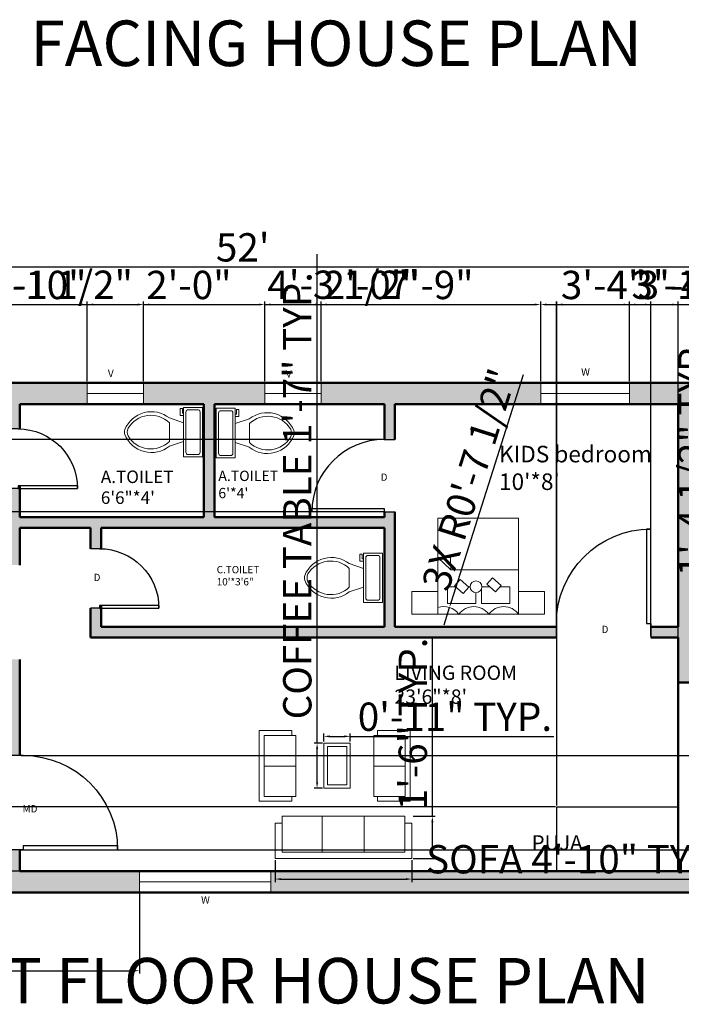
# Model space of a CAD drawing. Units: inches. Extents: x 2225 to 3094, y 1739 to 2599.
# Tile 3 of 5: x 2500 to 2780, y 2171 to 2588. Entities that reach past the tile are written whole.
import ezdxf

# ---------------------------------------------------------------- set-up
doc = ezdxf.new("R2010")
doc.units = ezdxf.units.IN
for name, color, linetype, lineweight in [('A-ANNO-DIMS', 2, 'Continuous', 18), ('A-ANNO-TEXT', 7, 'Continuous', 18), ('A-ANNO-TITL', 7, 'Continuous', 35), ('A-AREA-IDEN', 7, 'Continuous', 18), ('A-DOOR', 4, 'Continuous', 25), ('A-FLOR-CASE', 9, 'Continuous', 25), ('A-FLOR-FIXT', 9, 'Continuous', 18), ('A-FURN', 8, 'Continuous', 18), ('A-WALL-PATT', 160, 'Continuous', 13), ('WALL', 7, 'Continuous', 50), ('WINDOW', 130, 'Continuous', 18)]:
    doc.layers.add(name, color=color, linetype=linetype, lineweight=lineweight)
doc.styles.get("Standard").update_dxf_attribs({"font": 'arial.ttf'})
doc.dimstyles.new('ISO-25', dxfattribs={"dimtxt": 12, "dimasz": 2.5, "dimexe": 1.25, "dimexo": 0.625, "dimtad": 1, "dimdec": 0, "dimlunit": 4, "dimtxsty": 'Standard', "dimcen": 2.5, "dimadec": 0, "dimazin": 0, "dimtfac": 1, "dimtdec": 0, "dimtmove": 0, "dimatfit": 3, "dimfxl": 1, "dimarcsym": 0})

# ---------------------------------------------------------------- blocks, each defined once
blk = doc.blocks.new('*U2')
for p, q in [((9.5, -6), (9.5, -2)), ((-8, -8.5), (-8, -8)), ((-7, -8), (-7, -9.5)), ((-4, -8), (-6, -14)), ((4, -8), (6, -14)), ((-10, -8.5), (-8, -8.5)), ((-10, -9.5), (-10, -8.5)), ((-7, -9.5), (-10, -9.5)), ((4, -14), (-4, -14))]:
    blk.add_line(p, q)
blk.add_lwpolyline([(10.5, -8), (10.5, 0), (-10.5, 0), (-10.5, -8)], close=True)
for points in [[(-9.5, -2), (-9.5, -6)], [(8.5, -1), (-8.5, -1)], [(-8.5, -7), (8.5, -7)]]:
    blk.add_lwpolyline(points)
for centre, radius, start, end in [((-8.62, -1.88), 0.884, 81.8699, 188.1301), ((8.62, -1.88), 0.884, 351.8699, 98.1301), ((-8.62, -6.12), 0.884, 171.8699, 278.1301), ((8.62, -6.12), 0.884, 261.8699, 8.1301), ((3.52, -21.58), 12.17, 141.4691, 247.9714), ((4.2, -21.82), 11.33, 136.3677, 238.9468), ((-3.52, -21.58), 12.17, 292.0284, 38.5307), ((-4.2, -21.82), 11.33, 301.053, 43.6321), ((0, -27.88), 4, 245.7318, 294.2682), ((0, -29), 4, 254.8605, 285.1395)]:
    blk.add_arc(centre, radius, start, end)
blk = doc.blocks.new('*U4')
for p, q in [((0, 0), (0, -6)), ((40, 0), (40, -6))]:
    blk.add_line(p, q)
blk.add_lwpolyline([(0, 0), (0, 40), (1.75, 40), (1.75, 0)], close=True)
blk.add_arc((0, 0), 40, 0, 90)
blk = doc.blocks.new('*D5')
at = {"layer": 'A-ANNO-DIMS', "color": 0, "lineweight": -2, "transparency": 16777216}
for p, q in [((2282.56, 2434.95), (2282.56, 2484.67)), ((2285.06, 2483.42), (2904.06, 2483.42)), ((2906.56, 2434.95), (2906.56, 2484.67))]:
    blk.add_line(p, q, dxfattribs=at)
at = {"layer": 'A-ANNO-DIMS', "color": 0, "transparency": 16777216}
for points in [[(2285.06, 2483.83), (2285.06, 2483), (2282.56, 2483.42)], [(2904.06, 2483.83), (2904.06, 2483), (2906.56, 2483.42)]]:
    blk.add_solid(points, dxfattribs=at)
at = {"layer": 'Defpoints', "color": 0, "transparency": 16777216}
for p in [(2906.56, 2483.42), (2282.56, 2434.33), (2906.56, 2434.33)]:
    blk.add_point(p, dxfattribs=at)
at = {"layer": 'A-ANNO-DIMS', "color": 0, "transparency": 16777216, "insert": (2594.56, 2490.17), "char_height": 12, "attachment_point": 5}
blk.add_mtext("52'", dxfattribs=at)
blk = doc.blocks.new('BED-SINGLE')
for p, q in [((16.5, 18.81), (10.96, 24.02)), ((10.96, 24.02), (16.28, 24.02)), ((16.28, 24.02), (16.5, 18.81)), ((45.21, 18.81), (16.5, 18.81))]:
    blk.add_line(p, q)
for points in [[(45.21, 0), (45.21, 40.75), (10.96, 40.75), (10.96, 0)], [(21.65, 8.84), (18.05, 12.11), (20.5, 14.81), (24.1, 11.54)], [(35.37, 9.52), (31.76, 12.79), (34.21, 15.49), (37.82, 12.22)], [(10.96, 0), (10.96, 9.73), (0, 9.73), (0, 0)], [(56.18, 0), (56.18, 9.73), (45.21, 9.73), (45.21, 0)]]:
    blk.add_lwpolyline(points, close=True)
for points in [[(18.53, 11.67), (15.12, 11.67), (15.12, 4.64), (27.15, 4.64), (27.15, 9.17)], [(24.65, 11.67), (23.96, 11.67)], [(29.45, 10.68), (29.45, 4.64), (41.48, 4.64), (41.48, 11.67), (37.32, 11.67)], [(32.99, 11.67), (29.65, 11.67)]]:
    blk.add_lwpolyline(points)
blk.add_circle((27.15, 11.67), 2.5)
for centre, end in [((13.6, -4.42), 109.9878), ((26.25, -4.42), 145.0719), ((38.89, -4.42), 145.0719)]:
    blk.add_arc(centre, 7.71, 34.9281, end)
blk = doc.blocks.new('SOFA-THREE-SEAT')
for p, q in [((19.92, 17.92), (19.92, 2.75)), ((37.66, 17.92), (37.66, 2.75)), ((3.02, 14.97), (0, 14.97)), ((0, 14.97), (0, 0)), ((57.91, 14.97), (54.99, 14.97)), ((57.91, 0), (57.91, 14.97)), ((0, 0), (57.91, 0))]:
    blk.add_line(p, q)
blk.add_lwpolyline([(3.02, 2.75), (54.99, 2.75), (54.99, 17.92), (3.02, 17.92)], close=True)
blk = doc.blocks.new('SOFA-TWO-SEAT')
for p, q in [((1.66, 27.74), (1.66, 29.95)), ((1.66, 29.95), (15.43, 29.95)), ((15.43, 29.95), (15.43, 0)), ((0, 14.84), (13.39, 14.84)), ((1.66, 0), (1.66, 1.94)), ((15.43, 0), (1.66, 0))]:
    blk.add_line(p, q)
blk.add_lwpolyline([(13.39, 1.94), (0, 1.94), (0, 27.74), (13.39, 27.74)], close=True)
blk = doc.blocks.new('TABLE-COFFEE')
for points in [[(0, 0), (11.17, 0), (11.17, 19.11), (0, 19.11)], [(1.5, 1.5), (9.67, 1.5), (9.67, 17.61), (1.5, 17.61)]]:
    blk.add_lwpolyline(points, close=True)
blk = doc.blocks.new('WIN-55P7IN')
blk.add_line((0, 4.5), (55.68, 4.5))
blk.add_lwpolyline([(0, 0), (55.68, 0), (55.68, 9), (0, 9)], close=True)
blk = doc.blocks.new('*D32')
at = {"layer": 'A-ANNO-DIMS', "color": 0, "lineweight": -2, "transparency": 16777216}
for p, q in [((2608.3, 2232.07), (2608.3, 2222.75)), ((2666.2, 2232.07), (2666.2, 2222.75)), ((2610.8, 2224), (2663.7, 2224)), ((2666.2, 2224), (2802.66, 2224))]:
    blk.add_line(p, q, dxfattribs=at)
at = {"layer": 'A-ANNO-DIMS', "color": 0, "transparency": 16777216}
for points in [[(2610.8, 2224.42), (2610.8, 2223.59), (2608.3, 2224)], [(2663.7, 2224.42), (2663.7, 2223.59), (2666.2, 2224)]]:
    blk.add_solid(points, dxfattribs=at)
at = {"layer": 'Defpoints', "color": 0, "transparency": 16777216}
for p in [(2608.3, 2232.69), (2666.2, 2232.69), (2666.2, 2224)]:
    blk.add_point(p, dxfattribs=at)
at = {"layer": 'A-ANNO-DIMS', "color": 0, "transparency": 16777216, "insert": (2735.68, 2230.84), "char_height": 12, "attachment_point": 5}
blk.add_mtext('SOFA 4\'-10" TYP.', dxfattribs=at)
blk = doc.blocks.new('*D33')
at = {"layer": 'A-ANNO-DIMS', "color": 0, "lineweight": -2, "transparency": 16777216}
for p, q in [((2674.89, 2250.61), (2674.89, 2326.38)), ((2666.83, 2250.61), (2676.14, 2250.61)), ((2674.89, 2235.19), (2674.89, 2248.11)), ((2666.83, 2232.69), (2676.14, 2232.69))]:
    blk.add_line(p, q, dxfattribs=at)
at = {"layer": 'A-ANNO-DIMS', "color": 0, "transparency": 16777216}
for points in [[(2674.47, 2248.11), (2675.31, 2248.11), (2674.89, 2250.61)], [(2674.47, 2235.19), (2675.31, 2235.19), (2674.89, 2232.69)]]:
    blk.add_solid(points, dxfattribs=at)
at = {"layer": 'Defpoints', "color": 0, "transparency": 16777216}
for p in [(2666.2, 2250.61), (2674.89, 2250.61), (2666.2, 2232.69)]:
    blk.add_point(p, dxfattribs=at)
at = {"layer": 'A-ANNO-DIMS', "color": 0, "transparency": 16777216, "insert": (2668.14, 2289.74), "char_height": 12, "attachment_point": 5, "rotation": 90}
blk.add_mtext('1\'-6" TYP.', dxfattribs=at)
blk = doc.blocks.new('*D36')
at = {"layer": 'A-ANNO-DIMS', "color": 0, "lineweight": -2, "transparency": 16777216}
for p, q in [((2626.06, 2281.62), (2626.06, 2488.79)), ((2628.3, 2281.62), (2624.81, 2281.62)), ((2626.06, 2265.01), (2626.06, 2279.12)), ((2628.3, 2262.51), (2624.81, 2262.51))]:
    blk.add_line(p, q, dxfattribs=at)
at = {"layer": 'A-ANNO-DIMS', "color": 0, "transparency": 16777216}
for points in [[(2625.65, 2279.12), (2626.48, 2279.12), (2626.06, 2281.62)], [(2625.65, 2265.01), (2626.48, 2265.01), (2626.06, 2262.51)]]:
    blk.add_solid(points, dxfattribs=at)
at = {"layer": 'Defpoints', "color": 0, "transparency": 16777216}
for p in [(2626.06, 2281.62), (2628.93, 2281.62), (2628.93, 2262.51)]:
    blk.add_point(p, dxfattribs=at)
at = {"layer": 'A-ANNO-DIMS', "color": 0, "transparency": 16777216, "insert": (2619.23, 2386.46), "char_height": 12, "attachment_point": 5, "rotation": 90}
blk.add_mtext('COFFEE TABLE 1\'-7" TYP.', dxfattribs=at)
blk = doc.blocks.new('*D37')
at = {"layer": 'A-ANNO-DIMS', "color": 0, "lineweight": -2, "transparency": 16777216}
for p, q in [((2628.93, 2282.25), (2628.93, 2285.74)), ((2631.43, 2284.49), (2637.6, 2284.49)), ((2640.1, 2282.25), (2640.1, 2285.74)), ((2640.1, 2284.49), (2726.32, 2284.49))]:
    blk.add_line(p, q, dxfattribs=at)
at = {"layer": 'A-ANNO-DIMS', "color": 0, "transparency": 16777216}
for points in [[(2631.43, 2284.9), (2631.43, 2284.07), (2628.93, 2284.49)], [(2637.6, 2284.9), (2637.6, 2284.07), (2640.1, 2284.49)]]:
    blk.add_solid(points, dxfattribs=at)
at = {"layer": 'Defpoints', "color": 0, "transparency": 16777216}
for p in [(2640.1, 2284.49), (2628.93, 2281.62), (2640.1, 2281.62)]:
    blk.add_point(p, dxfattribs=at)
at = {"layer": 'A-ANNO-DIMS', "color": 0, "transparency": 16777216, "insert": (2684.46, 2291.24), "char_height": 12, "attachment_point": 5}
blk.add_mtext('0\'-11" TYP.', dxfattribs=at)
blk = doc.blocks.new('*D39')
at = {"layer": 'A-ANNO-DIMS', "color": 0, "lineweight": -2, "transparency": 16777216}
for p, q in [((2793.48, 2349.95), (2793.48, 2453.67)), ((2796.79, 2349.95), (2792.23, 2349.95)), ((2793.48, 2335.78), (2793.48, 2347.45)), ((2796.79, 2333.28), (2792.23, 2333.28))]:
    blk.add_line(p, q, dxfattribs=at)
at = {"layer": 'A-ANNO-DIMS', "color": 0, "transparency": 16777216}
for points in [[(2793.06, 2347.45), (2793.89, 2347.45), (2793.48, 2349.95)], [(2793.06, 2335.78), (2793.89, 2335.78), (2793.48, 2333.28)]]:
    blk.add_solid(points, dxfattribs=at)
at = {"layer": 'Defpoints', "color": 0, "transparency": 16777216}
for p in [(2793.48, 2349.95), (2797.42, 2349.95), (2797.42, 2333.28)]:
    blk.add_point(p, dxfattribs=at)
at = {"layer": 'A-ANNO-DIMS', "color": 0, "transparency": 16777216, "insert": (2786.65, 2403.06), "char_height": 12, "attachment_point": 5, "rotation": 90}
blk.add_mtext('1\'-4 1/2" TYP.', dxfattribs=at)
blk = doc.blocks.new('*D55')
at = {"layer": 'A-ANNO-DIMS', "color": 0, "lineweight": -2, "transparency": 16777216}
for p, q in [((2445.16, 2434.95), (2445.16, 2468.73)), ((2447.66, 2467.48), (2480.26, 2467.48)), ((2482.76, 2434.95), (2482.76, 2468.73)), ((2482.76, 2467.48), (2546.36, 2467.48))]:
    blk.add_line(p, q, dxfattribs=at)
at = {"layer": 'A-ANNO-DIMS', "color": 0, "transparency": 16777216}
for points in [[(2447.66, 2467.89), (2447.66, 2467.06), (2445.16, 2467.48)], [(2480.26, 2467.89), (2480.26, 2467.06), (2482.76, 2467.48)]]:
    blk.add_solid(points, dxfattribs=at)
at = {"layer": 'Defpoints', "color": 0, "transparency": 16777216}
for p in [(2482.76, 2467.48), (2445.16, 2434.33), (2482.76, 2434.33)]:
    blk.add_point(p, dxfattribs=at)
at = {"layer": 'A-ANNO-DIMS', "color": 0, "transparency": 16777216, "insert": (2515.81, 2474.31), "char_height": 12, "attachment_point": 5}
blk.add_mtext('3\'-1 1/2"', dxfattribs=at)
blk = doc.blocks.new('*D56')
at = {"layer": 'A-ANNO-DIMS', "color": 0, "lineweight": -2, "transparency": 16777216}
for p, q in [((2482.76, 2434.95), (2482.76, 2468.73)), ((2485.26, 2467.48), (2526.19, 2467.48)), ((2528.69, 2434.95), (2528.69, 2468.73))]:
    blk.add_line(p, q, dxfattribs=at)
at = {"layer": 'A-ANNO-DIMS', "color": 0, "transparency": 16777216}
for points in [[(2485.26, 2467.89), (2485.26, 2467.06), (2482.76, 2467.48)], [(2526.19, 2467.89), (2526.19, 2467.06), (2528.69, 2467.48)]]:
    blk.add_solid(points, dxfattribs=at)
at = {"layer": 'Defpoints', "color": 0, "transparency": 16777216}
for p in [(2528.69, 2467.48), (2482.76, 2434.33), (2528.69, 2434.33)]:
    blk.add_point(p, dxfattribs=at)
at = {"layer": 'A-ANNO-DIMS', "color": 0, "transparency": 16777216, "insert": (2505.72, 2474.23), "char_height": 12, "attachment_point": 5}
blk.add_mtext('3\'-10"', dxfattribs=at)
blk = doc.blocks.new('*D57')
at = {"layer": 'A-ANNO-DIMS', "color": 0, "lineweight": -2, "transparency": 16777216}
for p, q in [((2528.69, 2434.95), (2528.69, 2468.73)), ((2531.19, 2467.48), (2550.05, 2467.48)), ((2552.55, 2434.95), (2552.55, 2468.73)), ((2552.55, 2467.48), (2588.4, 2467.48))]:
    blk.add_line(p, q, dxfattribs=at)
at = {"layer": 'A-ANNO-DIMS', "color": 0, "transparency": 16777216}
for points in [[(2531.19, 2467.89), (2531.19, 2467.06), (2528.69, 2467.48)], [(2550.05, 2467.89), (2550.05, 2467.06), (2552.55, 2467.48)]]:
    blk.add_solid(points, dxfattribs=at)
at = {"layer": 'Defpoints', "color": 0, "transparency": 16777216}
for p in [(2552.55, 2467.48), (2528.69, 2434.33), (2552.55, 2434.33)]:
    blk.add_point(p, dxfattribs=at)
at = {"layer": 'A-ANNO-DIMS', "color": 0, "transparency": 16777216, "insert": (2571.73, 2474.23), "char_height": 12, "attachment_point": 5}
blk.add_mtext('2\'-0"', dxfattribs=at)
blk = doc.blocks.new('*D58')
at = {"layer": 'A-ANNO-DIMS', "color": 0, "lineweight": -2, "transparency": 16777216}
for p, q in [((2552.55, 2434.95), (2552.55, 2468.73)), ((2555.05, 2467.48), (2601.38, 2467.48)), ((2603.88, 2434.95), (2603.88, 2468.73)), ((2603.88, 2467.48), (2667.97, 2467.48))]:
    blk.add_line(p, q, dxfattribs=at)
at = {"layer": 'A-ANNO-DIMS', "color": 0, "transparency": 16777216}
for points in [[(2555.05, 2467.89), (2555.05, 2467.06), (2552.55, 2467.48)], [(2601.38, 2467.89), (2601.38, 2467.06), (2603.88, 2467.48)]]:
    blk.add_solid(points, dxfattribs=at)
at = {"layer": 'Defpoints', "color": 0, "transparency": 16777216}
for p in [(2603.88, 2467.48), (2552.55, 2434.33), (2603.88, 2434.33)]:
    blk.add_point(p, dxfattribs=at)
at = {"layer": 'A-ANNO-DIMS', "color": 0, "transparency": 16777216, "insert": (2637.18, 2474.31), "char_height": 12, "attachment_point": 5}
blk.add_mtext('4\'-3 1/2"', dxfattribs=at)
blk = doc.blocks.new('*D59')
at = {"layer": 'A-ANNO-DIMS', "color": 0, "lineweight": -2, "transparency": 16777216}
for p, q in [((2603.88, 2434.95), (2603.88, 2468.73)), ((2606.38, 2467.48), (2625.24, 2467.48)), ((2627.74, 2434.95), (2627.74, 2468.73)), ((2627.74, 2467.48), (2663.6, 2467.48))]:
    blk.add_line(p, q, dxfattribs=at)
at = {"layer": 'A-ANNO-DIMS', "color": 0, "transparency": 16777216}
for points in [[(2606.38, 2467.89), (2606.38, 2467.06), (2603.88, 2467.48)], [(2625.24, 2467.89), (2625.24, 2467.06), (2627.74, 2467.48)]]:
    blk.add_solid(points, dxfattribs=at)
at = {"layer": 'Defpoints', "color": 0, "transparency": 16777216}
for p in [(2627.74, 2467.48), (2603.88, 2434.33), (2627.74, 2434.33)]:
    blk.add_point(p, dxfattribs=at)
at = {"layer": 'A-ANNO-DIMS', "color": 0, "transparency": 16777216, "insert": (2646.92, 2474.23), "char_height": 12, "attachment_point": 5}
blk.add_mtext('2\'-0"', dxfattribs=at)
blk = doc.blocks.new('*D60')
at = {"layer": 'A-ANNO-DIMS', "color": 0, "lineweight": -2, "transparency": 16777216}
for p, q in [((2627.74, 2434.95), (2627.74, 2468.73)), ((2630.24, 2467.48), (2718.29, 2467.48)), ((2720.79, 2434.95), (2720.79, 2468.73))]:
    blk.add_line(p, q, dxfattribs=at)
at = {"layer": 'A-ANNO-DIMS', "color": 0, "transparency": 16777216}
for points in [[(2630.24, 2467.89), (2630.24, 2467.06), (2627.74, 2467.48)], [(2718.29, 2467.89), (2718.29, 2467.06), (2720.79, 2467.48)]]:
    blk.add_solid(points, dxfattribs=at)
at = {"layer": 'Defpoints', "color": 0, "transparency": 16777216}
for p in [(2720.79, 2467.48), (2627.74, 2434.33), (2720.79, 2434.33)]:
    blk.add_point(p, dxfattribs=at)
at = {"layer": 'A-ANNO-DIMS', "color": 0, "transparency": 16777216, "insert": (2674.27, 2474.23), "char_height": 12, "attachment_point": 5}
blk.add_mtext('7\'-9"', dxfattribs=at)
blk = doc.blocks.new('*D61')
at = {"layer": 'A-ANNO-DIMS', "color": 0, "lineweight": -2, "transparency": 16777216}
for p, q in [((2720.79, 2434.95), (2720.79, 2468.73)), ((2723.29, 2467.48), (2755.89, 2467.48)), ((2758.39, 2434.95), (2758.39, 2468.73)), ((2758.39, 2467.48), (2821.99, 2467.48))]:
    blk.add_line(p, q, dxfattribs=at)
at = {"layer": 'A-ANNO-DIMS', "color": 0, "transparency": 16777216}
for points in [[(2723.29, 2467.89), (2723.29, 2467.06), (2720.79, 2467.48)], [(2755.89, 2467.89), (2755.89, 2467.06), (2758.39, 2467.48)]]:
    blk.add_solid(points, dxfattribs=at)
at = {"layer": 'Defpoints', "color": 0, "transparency": 16777216}
for p in [(2758.39, 2467.48), (2720.79, 2434.33), (2758.39, 2434.33)]:
    blk.add_point(p, dxfattribs=at)
at = {"layer": 'A-ANNO-DIMS', "color": 0, "transparency": 16777216, "insert": (2791.44, 2474.31), "char_height": 12, "attachment_point": 5}
blk.add_mtext('3\'-1 1/2"', dxfattribs=at)
blk = doc.blocks.new('*D62')
at = {"layer": 'A-ANNO-DIMS', "color": 0, "lineweight": -2, "transparency": 16777216}
for p, q in [((2758.39, 2434.95), (2758.39, 2468.73)), ((2760.89, 2467.48), (2799.04, 2467.48)), ((2801.54, 2434.95), (2801.54, 2468.73))]:
    blk.add_line(p, q, dxfattribs=at)
at = {"layer": 'A-ANNO-DIMS', "color": 0, "transparency": 16777216}
for points in [[(2760.89, 2467.89), (2760.89, 2467.06), (2758.39, 2467.48)], [(2799.04, 2467.89), (2799.04, 2467.06), (2801.54, 2467.48)]]:
    blk.add_solid(points, dxfattribs=at)
at = {"layer": 'Defpoints', "color": 0, "transparency": 16777216}
for p in [(2801.54, 2467.48), (2758.39, 2434.33), (2801.54, 2434.33)]:
    blk.add_point(p, dxfattribs=at)
at = {"layer": 'A-ANNO-DIMS', "color": 0, "transparency": 16777216, "insert": (2779.97, 2474.23), "char_height": 12, "attachment_point": 5}
blk.add_mtext('3\'-7"', dxfattribs=at)
blk = doc.blocks.new('*D66')
at = {"layer": 'A-ANNO-DIMS', "color": 0, "lineweight": -2, "transparency": 16777216}
for p, q in [((2282.56, 2217.7), (2282.56, 2183.93)), ((2550.8, 2217.7), (2550.8, 2183.93)), ((2285.06, 2185.18), (2548.3, 2185.18))]:
    blk.add_line(p, q, dxfattribs=at)
at = {"layer": 'A-ANNO-DIMS', "color": 0, "transparency": 16777216}
for points in [[(2285.06, 2185.59), (2285.06, 2184.76), (2282.56, 2185.18)], [(2548.3, 2185.59), (2548.3, 2184.76), (2550.8, 2185.18)]]:
    blk.add_solid(points, dxfattribs=at)
at = {"layer": 'Defpoints', "color": 0, "transparency": 16777216}
for p in [(2282.56, 2218.33), (2550.8, 2218.33), (2550.8, 2185.18)]:
    blk.add_point(p, dxfattribs=at)
at = {"layer": 'A-ANNO-DIMS', "color": 0, "transparency": 16777216, "insert": (2416.68, 2191.83), "char_height": 12, "attachment_point": 5}
blk.add_mtext('22\'-4"', dxfattribs=at)
blk = doc.blocks.new('*D68')
at = {"layer": 'A-ANNO-DIMS', "color": 0, "lineweight": -2, "transparency": 16777216}
for p, q in [((2500.68, 2276.4), (2940.96, 2276.4)), ((2939.71, 2273.9), (2939.71, 2238.9)), ((2500.68, 2236.4), (2940.96, 2236.4))]:
    blk.add_line(p, q, dxfattribs=at)
at = {"layer": 'A-ANNO-DIMS', "color": 0, "transparency": 16777216}
for points in [[(2939.29, 2273.9), (2940.12, 2273.9), (2939.71, 2276.4)], [(2939.29, 2238.9), (2940.12, 2238.9), (2939.71, 2236.4)]]:
    blk.add_solid(points, dxfattribs=at)
at = {"layer": 'Defpoints', "color": 0, "transparency": 16777216}
for p in [(2500.06, 2276.4), (2500.06, 2236.4), (2939.71, 2236.4)]:
    blk.add_point(p, dxfattribs=at)
at = {"layer": 'A-ANNO-DIMS', "color": 0, "transparency": 16777216, "insert": (2932.95, 2256.4), "char_height": 12, "attachment_point": 5, "rotation": 90}
blk.add_mtext('3\'-4"', dxfattribs=at)
blk = doc.blocks.new('*D70')
at = {"layer": 'A-ANNO-DIMS', "color": 0, "lineweight": -2, "transparency": 16777216}
for p, q in [((2727.43, 2326.95), (2727.43, 2468.73)), ((2729.93, 2467.48), (2764.93, 2467.48)), ((2767.43, 2326.95), (2767.43, 2468.73))]:
    blk.add_line(p, q, dxfattribs=at)
at = {"layer": 'A-ANNO-DIMS', "color": 0, "transparency": 16777216}
for points in [[(2729.93, 2467.89), (2729.93, 2467.06), (2727.43, 2467.48)], [(2764.93, 2467.89), (2764.93, 2467.06), (2767.43, 2467.48)]]:
    blk.add_solid(points, dxfattribs=at)
at = {"layer": 'Defpoints', "color": 0, "transparency": 16777216}
for p in [(2767.43, 2467.48), (2727.43, 2326.33), (2767.43, 2326.33)]:
    blk.add_point(p, dxfattribs=at)
at = {"layer": 'A-ANNO-DIMS', "color": 0, "transparency": 16777216, "insert": (2747.43, 2474.23), "char_height": 12, "attachment_point": 5}
blk.add_mtext('3\'-4"', dxfattribs=at)
blk = doc.blocks.new('*D72')
at = {"layer": 'A-ANNO-DIMS', "color": 0, "lineweight": -2, "transparency": 16777216}
for p, q in [((2249.41, 2410.28), (2249.41, 2474.1)), ((2653.84, 2410.28), (2248.16, 2410.28)), ((2249.41, 2382.17), (2249.41, 2407.78)), ((2653.84, 2379.67), (2248.16, 2379.67))]:
    blk.add_line(p, q, dxfattribs=at)
at = {"layer": 'A-ANNO-DIMS', "color": 0, "transparency": 16777216}
for points in [[(2248.99, 2407.78), (2249.82, 2407.78), (2249.41, 2410.28)], [(2248.99, 2382.17), (2249.82, 2382.17), (2249.41, 2379.67)]]:
    blk.add_solid(points, dxfattribs=at)
at = {"layer": 'Defpoints', "color": 0, "transparency": 16777216}
for p in [(2249.41, 2410.28), (2654.47, 2410.28), (2654.47, 2379.67)]:
    blk.add_point(p, dxfattribs=at)
at = {"layer": 'A-ANNO-DIMS', "color": 0, "transparency": 16777216, "insert": (2242.58, 2443.44), "char_height": 12, "attachment_point": 5, "rotation": 90}
blk.add_mtext('2\'-6 1/2"', dxfattribs=at)
blk = doc.blocks.new('*D74')
at = {"layer": 'A-ANNO-DIMS', "color": 0, "lineweight": -2, "transparency": 16777216}
for p, q in [((2727.64, 2255.24), (2727.64, 2468.73)), ((2730.14, 2467.48), (2776.56, 2467.48)), ((2779.06, 2255.24), (2779.06, 2468.73)), ((2779.06, 2467.48), (2843.15, 2467.48))]:
    blk.add_line(p, q, dxfattribs=at)
at = {"layer": 'A-ANNO-DIMS', "color": 0, "transparency": 16777216}
for points in [[(2730.14, 2467.89), (2730.14, 2467.06), (2727.64, 2467.48)], [(2776.56, 2467.89), (2776.56, 2467.06), (2779.06, 2467.48)]]:
    blk.add_solid(points, dxfattribs=at)
at = {"layer": 'Defpoints', "color": 0, "transparency": 16777216}
for p in [(2779.06, 2467.48), (2727.64, 2254.61), (2779.06, 2254.61)]:
    blk.add_point(p, dxfattribs=at)
at = {"layer": 'A-ANNO-DIMS', "color": 0, "transparency": 16777216, "insert": (2812.35, 2474.31), "char_height": 12, "attachment_point": 5}
blk.add_mtext('4\'-3 1/2"', dxfattribs=at)
blk = doc.blocks.new('*D75')
at = {"layer": 'A-ANNO-DIMS', "color": 0, "lineweight": -2, "transparency": 16777216}
for p, q in [((2249.41, 2254.61), (2249.41, 2318.43)), ((2727.01, 2254.61), (2248.16, 2254.61)), ((2249.41, 2229.83), (2249.41, 2252.11)), ((2727.01, 2227.33), (2248.16, 2227.33))]:
    blk.add_line(p, q, dxfattribs=at)
at = {"layer": 'A-ANNO-DIMS', "color": 0, "transparency": 16777216}
for points in [[(2248.99, 2252.11), (2249.82, 2252.11), (2249.41, 2254.61)], [(2248.99, 2229.83), (2249.82, 2229.83), (2249.41, 2227.33)]]:
    blk.add_solid(points, dxfattribs=at)
at = {"layer": 'Defpoints', "color": 0, "transparency": 16777216}
for p in [(2249.41, 2254.61), (2727.64, 2254.61), (2727.64, 2227.33)]:
    blk.add_point(p, dxfattribs=at)
at = {"layer": 'A-ANNO-DIMS', "color": 0, "transparency": 16777216, "insert": (2242.57, 2287.77), "char_height": 12, "attachment_point": 5, "rotation": 90}
blk.add_mtext('2\'-3 1/2"', dxfattribs=at)
blk = doc.blocks.new('*D81')
at = {"layer": 'A-ANNO-DIMS', "color": 0, "lineweight": -2, "transparency": 16777216}
for p, q in [((2713.3, 2437.7), (2682.91, 2341.52)), ((2679.83, 2331.78), (2682.15, 2339.14))]:
    blk.add_line(p, q, dxfattribs=at)
at = {"layer": 'A-ANNO-DIMS', "color": 0, "transparency": 16777216}
blk.add_solid([(2682.51, 2341.65), (2683.3, 2341.39), (2682.15, 2339.14)], dxfattribs=at)
at = {"layer": 'Defpoints', "color": 0, "transparency": 16777216}
for p in [(2682.15, 2339.14), (2679.83, 2331.78)]:
    blk.add_point(p, dxfattribs=at)
at = {"layer": 'A-ANNO-DIMS', "color": 0, "transparency": 16777216, "insert": (2691.97, 2392.86), "char_height": 12, "attachment_point": 5, "rotation": 72.4604}
blk.add_mtext('3X R0\'-7 1/2"', dxfattribs=at)

msp = doc.modelspace()

# ---------------------------------------------------------------- hatches: boundary and pattern name
at = {"layer": 'A-WALL-PATT'}
h = msp.add_hatch(color=256, dxfattribs=at)
h.dxf.hatch_style = 1
h.paths.add_polyline_path([(2445.16, 2434.33), (2282.56, 2434.33), (2282.56, 2366.97), (2291.56, 2366.97), (2291.56, 2425.33), (2445.16, 2425.33)], flags=17)
h.paths.add_polyline_path([(2528.69, 2434.33), (2482.76, 2434.33), (2482.76, 2425.33), (2495.56, 2425.33), (2495.56, 2414.78), (2499.34, 2414.78, -0.007163), (2500.06, 2414.76), (2500.06, 2425.33), (2528.69, 2425.33)], flags=17)
h.paths.add_polyline_path([(2867.81, 2330.83), (2783.56, 2330.83), (2783.56, 2354.83), (2783.56, 2425.33), (2801.54, 2425.33), (2801.54, 2434.33), (2758.39, 2434.33), (2758.39, 2425.33), (2779.06, 2425.33), (2779.06, 2330.83), (2767.43, 2330.83), (2767.43, 2326.33), (2779.06, 2326.33), (2779.06, 2307.37), (2783.56, 2307.37), (2783.56, 2326.33), (2867.81, 2326.33)])
h.paths.add_polyline_path([(2906.56, 2434.33), (2839.14, 2434.33), (2839.14, 2425.33), (2897.56, 2425.33), (2897.56, 2330.83), (2897.56, 2326.33), (2897.56, 2264.13), (2906.56, 2264.13)])
h.paths.add_polyline_path([(2906.56, 2236.32), (2897.56, 2236.32), (2897.56, 2227.33), (2860.08, 2227.33), (2860.08, 2218.33), (2906.56, 2218.33)])
h.paths.add_polyline_path([(2815.14, 2227.33), (2783.56, 2227.33), (2779.06, 2227.33), (2727.64, 2227.33), (2606.48, 2227.33), (2606.48, 2218.33), (2815.14, 2218.33)])
h.paths.add_polyline_path([(2780.45, 2273.09), (2785.35, 2273.09), (2785.35, 2279.46), (2780.45, 2279.46)], flags=9)
h.paths.add_polyline_path([(2500.16, 2250.57), (2508.42, 2250.57), (2508.42, 2256.93), (2500.16, 2256.93)], flags=25)
h.paths.add_polyline_path([(2745.49, 2326.59), (2750.15, 2326.59), (2750.15, 2332.96), (2745.49, 2332.96)], flags=9)
h.paths.add_polyline_path([(2651.86, 2391.09), (2656.53, 2391.09), (2656.53, 2397.46), (2651.86, 2397.46)], flags=9)
h.paths.add_polyline_path([(2493.47, 2330.16), (2498.13, 2330.16), (2498.13, 2336.53), (2493.47, 2336.53)], flags=25)
h.paths.add_polyline_path([(2530.27, 2348.62), (2534.93, 2348.62), (2534.93, 2354.99), (2530.27, 2354.99)], flags=25)
h.paths.add_polyline_path([(2432.89, 2282.56), (2450.26, 2282.56), (2450.26, 2294.09), (2432.89, 2294.09)], flags=25)
h.paths.add_polyline_path([(2735.79, 2240.68), (2748.37, 2240.68), (2748.37, 2247.05), (2735.79, 2247.05)], flags=9)
h.paths.add_polyline_path([(2717.02, 2288.94), (2747.35, 2288.94), (2747.35, 2300.47), (2717.02, 2300.47)], flags=9)
h.paths.add_polyline_path([(2839.5, 2270.61), (2856.29, 2270.61), (2856.29, 2282.14), (2839.5, 2282.14)], flags=25)
h.paths.add_polyline_path([(2825.64, 2385.51), (2846.28, 2385.51), (2846.28, 2397.04), (2825.64, 2397.04)], flags=25)
h.paths.add_polyline_path([(2692.05, 2396.34), (2722.05, 2396.34), (2722.05, 2407.87), (2692.05, 2407.87)], flags=9)
h.paths.add_polyline_path([(2282.56, 2366.97), (2291.56, 2366.97), (2291.56, 2425.33), (2445.16, 2425.33), (2445.16, 2434.33), (2282.56, 2434.33)])
h.paths.add_polyline_path([(2291.56, 2341.62), (2282.56, 2341.62), (2282.56, 2218.33), (2550.8, 2218.33), (2550.8, 2227.33), (2500.06, 2227.33), (2500.06, 2236.4), (2495.56, 2236.4), (2495.56, 2227.33), (2291.56, 2227.33), (2291.56, 2306.83), (2327.56, 2306.83), (2495.56, 2306.83), (2495.56, 2276.4), (2500.06, 2276.4), (2500.06, 2306.83), (2500.06, 2317.06), (2495.56, 2317.06), (2495.56, 2311.33), (2291.56, 2311.33)])
h = msp.add_hatch(color=256, dxfattribs=at)
h.dxf.hatch_style = 1
h.paths.add_polyline_path([(2727.43, 2330.83), (2659.06, 2330.83), (2659.06, 2379.67), (2654.56, 2379.67), (2654.56, 2377.33), (2582.56, 2377.33), (2582.56, 2425.33), (2603.88, 2425.33), (2603.88, 2434.33), (2552.55, 2434.33), (2552.55, 2425.33), (2578.06, 2425.33), (2578.06, 2377.33), (2500.06, 2377.33), (2500.06, 2389.59), (2499.34, 2389.59), (2495.56, 2389.59), (2495.56, 2357.06), (2500.06, 2357.06), (2500.06, 2372.83), (2530.06, 2372.83), (2530.06, 2364.02), (2533.84, 2364.02, -0.007163), (2534.56, 2364.01), (2534.56, 2372.83), (2578.06, 2372.83), (2582.56, 2372.83), (2654.56, 2372.83), (2654.56, 2330.83), (2582.56, 2330.83), (2581.71, 2330.83), (2578.06, 2330.83), (2534.56, 2330.83), (2534.56, 2338.83), (2533.84, 2338.83), (2530.06, 2338.83), (2530.06, 2326.33), (2659.06, 2326.33), (2727.43, 2326.33)])
h.paths.add_polyline_path([(2720.79, 2434.33), (2627.74, 2434.33), (2627.74, 2425.33), (2654.56, 2425.33), (2654.56, 2410.28), (2659.06, 2410.28), (2659.06, 2425.33), (2720.79, 2425.33)], flags=17)
h.paths.add_polyline_path([(2445.16, 2434.33), (2282.56, 2434.33), (2282.56, 2366.97), (2291.56, 2366.97), (2291.56, 2425.33), (2445.16, 2425.33)])

# ---------------------------------------------------------------- linework, layer by layer
at = {"layer": 'A-FLOR-CASE'}
msp.add_lwpolyline([(2779.06, 2227.33), (2727.64, 2227.33), (2727.64, 2254.61), (2779.06, 2254.61)], close=True, dxfattribs=at)
at = {"layer": 'WALL'}
for p, q in [((2500.06, 2425.33), (2500.06, 2414.76)), ((2500.06, 2425.33), (2500.06, 2414.76)), ((2578.06, 2425.33), (2578.06, 2377.33)), ((2582.56, 2425.33), (2582.56, 2377.33)), ((2654.56, 2425.33), (2654.56, 2410.28)), ((2659.06, 2425.33), (2659.06, 2410.28)), ((2779.06, 2425.33), (2779.06, 2330.83)), ((2500.06, 2390.69), (2500.06, 2377.33)), ((2500.06, 2390.69), (2500.06, 2377.33)), ((2654.56, 2379.67), (2654.56, 2377.33)), ((2659.06, 2379.67), (2659.06, 2330.83)), ((2500.06, 2377.33), (2578.06, 2377.33)), ((2582.56, 2377.33), (2654.56, 2377.33)), ((2500.06, 2372.83), (2530.06, 2372.83)), ((2500.06, 2372.83), (2500.06, 2357.06)), ((2530.06, 2364.02), (2530.06, 2372.83)), ((2534.56, 2372.83), (2578.06, 2372.83)), ((2534.56, 2364.01), (2534.56, 2372.83)), ((2578.06, 2372.83), (2582.56, 2372.83)), ((2582.56, 2372.83), (2654.56, 2372.83)), ((2654.56, 2372.83), (2654.56, 2330.83)), ((2654.56, 2372.83), (2654.56, 2330.83)), ((2530.06, 2326.33), (2530.06, 2338.83)), ((2534.56, 2330.83), (2534.56, 2339.93)), ((2578.06, 2330.83), (2534.56, 2330.83)), ((2578.06, 2330.83), (2581.71, 2330.83)), ((2581.71, 2330.83), (2584.98, 2330.83)), ((2654.56, 2330.83), (2582.56, 2330.83)), ((2659.06, 2330.83), (2727.43, 2330.83)), ((2767.43, 2330.83), (2779.06, 2330.83)), ((2659.06, 2326.33), (2530.06, 2326.33)), ((2659.06, 2326.33), (2727.43, 2326.33)), ((2767.43, 2326.33), (2779.06, 2326.33)), ((2779.06, 2326.33), (2779.06, 2227.33)), ((2500.06, 2317.06), (2500.06, 2306.83)), ((2500.06, 2306.83), (2500.06, 2276.4)), ((2779.06, 2307.37), (2783.56, 2307.37)), ((2500.06, 2236.4), (2500.06, 2227.33)), ((2779.06, 2227.33), (2777.56, 2227.33)), ((2779.06, 2227.33), (2783.56, 2227.33))]:
    msp.add_line(p, q, dxfattribs=at)
msp.add_lwpolyline([(2282.56, 2218.33), (2906.56, 2218.33), (2906.56, 2434.33), (2282.56, 2434.33)], close=True, dxfattribs=at)
for points in [[(2578.06, 2425.33), (2500.06, 2425.33)], [(2654.56, 2425.33), (2582.56, 2425.33)], [(2779.06, 2425.33), (2659.06, 2425.33)], [(2500.06, 2227.33), (2779.06, 2227.33)]]:
    msp.add_lwpolyline(points, dxfattribs=at)
at = {"layer": 'WINDOW'}
for p, q in [((2528.69, 2429.83), (2552.55, 2429.83)), ((2603.88, 2429.83), (2627.74, 2429.83)), ((2720.79, 2429.83), (2758.39, 2429.83))]:
    msp.add_line(p, q, dxfattribs=at)
for points in [[(2528.69, 2425.33), (2552.55, 2425.33), (2552.55, 2434.33), (2528.69, 2434.33)], [(2603.88, 2425.33), (2627.74, 2425.33), (2627.74, 2434.33), (2603.88, 2434.33)], [(2758.39, 2425.33), (2720.79, 2425.33), (2720.79, 2434.33), (2758.39, 2434.33)]]:
    msp.add_lwpolyline(points, close=True, dxfattribs=at)

# ---------------------------------------------------------------- block references
at = {"layer": 'A-DOOR'}
for p, xscale, yscale, zscale, rotation in [((2499.34, 2389.59), -0.6297308224195742, 0.6297308224195742, 0.6297308224195742, 270), ((2654.47, 2379.67), 0.7652481811317178, 0.7652481811317178, 0.7652481811317178, 89.99999999999999), ((2533.84, 2338.83), -0.6297308224195742, 0.6297308224195742, 0.6297308224195742, 270)]:
    msp.add_blockref('*U4', p, dxfattribs=dict(at, xscale=xscale, yscale=yscale, zscale=zscale, rotation=rotation))
at = {"layer": 'A-DOOR', "xscale": -1}
msp.add_blockref('*U4', (2767.43, 2332.33), dxfattribs=at)
at = {"layer": 'A-DOOR', "xscale": -1, "rotation": 270}
msp.add_blockref('*U4', (2501.56, 2236.4), dxfattribs=at)
at = {"layer": 'A-FLOR-FIXT', "rotation": 270}
for p in [(2577.48, 2413.42), (2653.71, 2351.67)]:
    msp.add_blockref('*U2', p, dxfattribs=at)
at = {"layer": 'A-FLOR-FIXT', "xscale": -1, "rotation": 90}
msp.add_blockref('*U2', (2583.35, 2413.01), dxfattribs=at)
at = {"layer": 'A-FURN'}
for name, p in [('BED-SINGLE', (2666.23, 2336.2)), ('SOFA-TWO-SEAT', (2650.04, 2257.06)), ('TABLE-COFFEE', (2628.93, 2262.51)), ('SOFA-THREE-SEAT', (2608.3, 2232.69))]:
    msp.add_blockref(name, p, dxfattribs=at)
at = {"layer": 'A-FURN', "extrusion": (0, 0, -1), "zscale": -1}
msp.add_blockref('SOFA-TWO-SEAT', (-2617.01, 2257.06), dxfattribs=at)
at = {"layer": 'WINDOW'}
msp.add_blockref('WIN-55P7IN', (2550.8, 2218.33), dxfattribs=at)

# ---------------------------------------------------------------- texts
at = {"layer": 'A-ANNO-TEXT', "char_height": 3.09, "attachment_point": 1}
for s, insert in [('V', (2537.44, 2439.82)), ('V', (2612.87, 2439.64)), ('W', (2737.94, 2440.44)), ('D', (2652.97, 2395.87)), ('D', (2531.37, 2353.4)), ('D', (2746.59, 2331.37)), ('MD', (2501.25, 2255.34)), ('W', (2576.91, 2216.72))]:
    msp.add_mtext_dynamic_manual_height_columns(s, width=49.525, gutter_width=15.45, heights=[0], dxfattribs=dict(at, insert=insert))
at = {"layer": 'A-ANNO-TITL', "char_height": 19.3093, "attachment_point": 1}
for s, insert in [('SOUTH FACING HOUSE PLAN', (2409.47, 2587.86)), ('FIRST FLOOR HOUSE PLAN', (2439.06, 2190.58))]:
    msp.add_mtext_dynamic_manual_height_columns(s, width=2944.6637, gutter_width=96.55, heights=[0], dxfattribs=dict(at, insert=insert))
at = {"layer": 'A-AREA-IDEN', "attachment_point": 1}
for s, width, gutter_width, insert, char_height in [("KIDS bedroom\\P10'*8'", 112.5018, 35.1, (2703.14, 2407.62), 7.0191), ('A.TOILET\\P6\'6"*4\'', 85.0926, 26.54, (2534.44, 2397.14), 5.309), ("A.TOILET\\P6'*4'", 70.1073, 21.87, (2584.21, 2397.07), 4.374), ('C.TOILET\\P10\'*3\'6"', 49.525, 15.45, (2583.52, 2356.69), 3.09), ('LIVING ROOM\\P23\'6"*8\'', 97.3586, 30.37, (2658.79, 2314.48), 6.0743), ('PUJA', 101.3669, 31.62, (2716.97, 2242.56), 6.324)]:
    msp.add_mtext_dynamic_manual_height_columns(s, width=width, gutter_width=gutter_width, heights=[0], dxfattribs=dict(at, insert=insert, char_height=char_height))

# ---------------------------------------------------------------- dimensions: what is measured, and where the dimension line sits
at = {"layer": 'A-ANNO-DIMS'}
for base, p1, p2, override, picture, middle in [((2906.56, 2483.42), (2282.56, 2434.33), (2906.56, 2434.33), {"dimclrd": 0, "dimclre": 0, "dimclrt": 0}, '*D5', (2594.56, 2490.17)), ((2482.76, 2467.48), (2445.16, 2434.33), (2482.76, 2434.33), {"dimdec": 1, "dimlfac": 1, "dimrnd": 0, "dimzin": 1, "dimdsep": 46, "dimlunit": 4, "dimfrac": 2}, '*D55', (2515.81, 2474.31)), ((2603.88, 2467.48), (2552.55, 2434.33), (2603.88, 2434.33), {"dimdec": 1, "dimlfac": 1, "dimrnd": 0, "dimzin": 1, "dimdsep": 46, "dimlunit": 4, "dimfrac": 2}, '*D58', (2637.18, 2474.31)), ((2758.39, 2467.48), (2720.79, 2434.33), (2758.39, 2434.33), {"dimdec": 1, "dimlfac": 1, "dimrnd": 0, "dimzin": 1, "dimdsep": 46, "dimlunit": 4, "dimfrac": 2}, '*D61', (2791.44, 2474.31)), ((2779.06, 2467.48), (2727.64, 2254.61), (2779.06, 2254.61), {"dimdec": 1, "dimlfac": 1, "dimrnd": 0, "dimzin": 1, "dimdsep": 46, "dimlunit": 4, "dimfrac": 2}, '*D74', (2812.35, 2474.31)), ((2528.69, 2467.48), (2482.76, 2434.33), (2528.69, 2434.33), {"dimdec": 1, "dimlfac": 1, "dimrnd": 0, "dimzin": 1, "dimdsep": 46, "dimlunit": 4, "dimfrac": 2}, '*D56', (2505.72, 2474.23)), ((2552.55, 2467.48), (2528.69, 2434.33), (2552.55, 2434.33), {"dimdec": 1, "dimlfac": 1, "dimrnd": 0, "dimzin": 1, "dimdsep": 46, "dimlunit": 4, "dimfrac": 2}, '*D57', (2571.73, 2474.23)), ((2627.74, 2467.48), (2603.88, 2434.33), (2627.74, 2434.33), {"dimdec": 1, "dimlfac": 1, "dimrnd": 0, "dimzin": 1, "dimdsep": 46, "dimlunit": 4, "dimfrac": 2}, '*D59', (2646.92, 2474.23)), ((2720.7934, 2467.4778), (2627.7418, 2434.3278), (2720.7934, 2434.3278), {"dimdec": 1, "dimlfac": 1, "dimrnd": 0, "dimzin": 1, "dimdsep": 46, "dimlunit": 4, "dimfrac": 2}, '*D60', (2674.2676, 2474.2296)), ((2767.43, 2467.48), (2727.43, 2326.33), (2767.43, 2326.33), {"dimdec": 1, "dimlfac": 1, "dimrnd": 0, "dimzin": 1, "dimdsep": 46, "dimlunit": 4, "dimfrac": 2}, '*D70', (2747.43, 2474.23)), ((2801.5388, 2467.4778), (2758.3918, 2434.3278), (2801.5388, 2434.3278), {"dimdec": 1, "dimlfac": 1, "dimrnd": 0, "dimzin": 1, "dimdsep": 46, "dimlunit": 4, "dimfrac": 2}, '*D62', (2779.9653, 2474.2337)), ((2550.8, 2185.18), (2282.56, 2218.33), (2550.8, 2218.33), {"dimdec": 1, "dimlfac": 1, "dimrnd": 0, "dimzin": 1, "dimdsep": 46, "dimlunit": 4, "dimfrac": 2}, '*D66', (2416.68, 2191.83))]:
    dim = msp.add_linear_dim(base=base, p1=p1, p2=p2, dimstyle='ISO-25', override=override, dxfattribs=at)
    dim.commit()
    dim.dimension.update_dxf_attribs({"geometry": picture, "text_midpoint": middle})
for base, p1, p2, text, picture, middle in [((2626.06, 2281.62), (2628.93, 2262.51), (2628.93, 2281.62), 'COFFEE TABLE <> TYP.', '*D36', (2619.23, 2386.46)), ((2793.48, 2349.95), (2797.42, 2333.28), (2797.42, 2349.95), '<> TYP.', '*D39', (2786.65, 2403.06)), ((2674.89, 2250.61), (2666.2, 2232.69), (2666.2, 2250.61), '<> TYP.', '*D33', (2668.14, 2289.74))]:
    dim = msp.add_linear_dim(base=base, p1=p1, p2=p2, angle=90, text=text, dimstyle='ISO-25', override={"dimdec": 1, "dimlfac": 1, "dimrnd": 0, "dimzin": 1, "dimdsep": 46, "dimlunit": 4, "dimfrac": 2}, dxfattribs=at)
    dim.commit()
    dim.dimension.update_dxf_attribs({"geometry": picture, "text_midpoint": middle})
for base, p1, p2, picture, middle in [((2249.41, 2410.28), (2654.47, 2379.67), (2654.47, 2410.28), '*D72', (2242.58, 2443.44)), ((2249.41, 2254.61), (2727.64, 2227.33), (2727.64, 2254.61), '*D75', (2242.57, 2287.77)), ((2939.71, 2236.4), (2500.06, 2276.4), (2500.06, 2236.4), '*D68', (2932.95, 2256.4))]:
    dim = msp.add_linear_dim(base=base, p1=p1, p2=p2, angle=90, dimstyle='ISO-25', override={"dimdec": 1, "dimlfac": 1, "dimrnd": 0, "dimzin": 1, "dimdsep": 46, "dimlunit": 4, "dimfrac": 2}, dxfattribs=at)
    dim.commit()
    dim.dimension.update_dxf_attribs({"geometry": picture, "text_midpoint": middle})
dim = msp.add_radius_dim(center=(2679.83, 2331.78), mpoint=(2682.15, 2339.14), text='3X <>', dimstyle='ISO-25', override={"dimdec": 1, "dimlfac": 1, "dimrnd": 0, "dimzin": 1, "dimdsep": 46, "dimlunit": 4, "dimfrac": 2}, dxfattribs=at)
dim.commit()
dim.dimension.update_dxf_attribs({"geometry": '*D81', "text_midpoint": (2691.97, 2392.86)})
for base, p1, p2, text, picture, middle in [((2640.1, 2284.49), (2628.93, 2281.62), (2640.1, 2281.62), '<> TYP.', '*D37', (2684.46, 2291.24)), ((2666.2, 2224), (2608.3, 2232.69), (2666.2, 2232.69), 'SOFA <> TYP.', '*D32', (2735.68, 2230.84))]:
    dim = msp.add_linear_dim(base=base, p1=p1, p2=p2, text=text, dimstyle='ISO-25', override={"dimdec": 1, "dimlfac": 1, "dimrnd": 0, "dimzin": 1, "dimdsep": 46, "dimlunit": 4, "dimfrac": 2}, dxfattribs=at)
    dim.commit()
    dim.dimension.update_dxf_attribs({"geometry": picture, "text_midpoint": middle})

doc.saveas('drawing.dxf')
